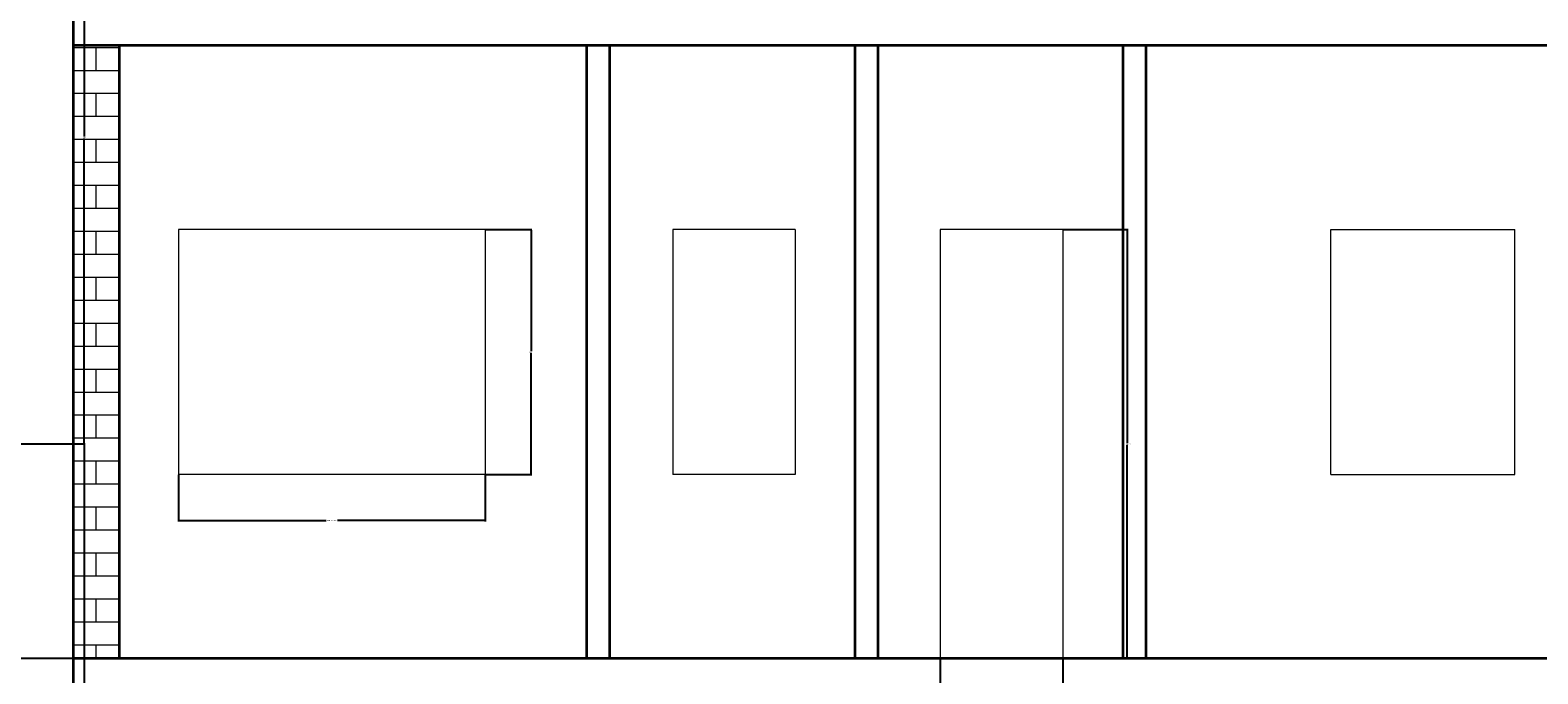
# Model space of a CAD drawing. Units: inches. Extents: x 2120 to 4013, y 1390 to 3019.
# Tile 56 of 59: x 3063 to 3358, y 2598 to 2724. Entities that reach past the tile are written whole.
import ezdxf

# ---------------------------------------------------------------- set-up
doc = ezdxf.new("R2010")
doc.units = ezdxf.units.IN
for name, color, linetype, lineweight in [('A-ANNO-DIMS', 2, 'Continuous', 18), ('A-DOOR', 3, 'Continuous', 18), ('A-GLAZ', 4, 'Continuous', 18), ('A-SECT', 7, 'Continuous', 35), ('A-WALL-PATT', 252, 'Continuous', 13)]:
    doc.layers.add(name, color=color, linetype=linetype, lineweight=lineweight)
doc.styles.get("Standard").update_dxf_attribs({"font": 'arial.ttf'})
doc.dimstyles.get("Standard").update_dxf_attribs({"dimtxt": 0.18, "dimasz": 0.18, "dimexe": 0.18, "dimexo": 0.0625, "dimgap": 0.09, "dimtad": 0, "dimtih": 1, "dimtoh": 1, "dimdec": 4, "dimzin": 0, "dimdsep": 46, "dimtxsty": 'Standard', "dimcen": 0.09, "dimadec": 0, "dimazin": 0, "dimtfac": 1, "dimtdec": 4, "dimtofl": 0, "dimtmove": 0, "dimatfit": 3, "dimfxl": 1, "dimtolj": 1, "dimtzin": 0, "dimarcsym": 0})

# ---------------------------------------------------------------- blocks, each defined once
blk = doc.blocks.new('WIN-SECT-60IN')
for p, q in [((0, 48), (0, 0)), ((60, 48), (0, 48)), ((60, 48), (60, 0)), ((60, 0), (0, 0))]:
    blk.add_line(p, q)
blk = doc.blocks.new('WIN-SECT-24IN')
for p, q in [((0, 48), (0, 0)), ((0, 48), (0, 0)), ((24, 48), (0, 48)), ((24, 48), (24, 0)), ((24, 0), (0, 0))]:
    blk.add_line(p, q)
blk = doc.blocks.new('DOOR-SECT-24IN')
for p, q in [((0, 84), (0, 0)), ((24, 84), (0, 84)), ((24, 84), (24, 0))]:
    blk.add_line(p, q)
blk = doc.blocks.new('WIN-SECT-36IN')
for p, q in [((0, 48), (0, 0)), ((36, 48), (0, 48)), ((36, 48), (36, 0)), ((36, 0), (0, 0))]:
    blk.add_line(p, q)
blk = doc.blocks.new('*D197')
at = {"layer": 'A-ANNO-DIMS', "color": 0, "lineweight": -2, "transparency": 16777216}
for p, q in [((3092.38, 2637.25), (3092.38, 2628.13)), ((3152.38, 2637.25), (3152.38, 2628.13)), ((3092.56, 2628.31), (3121.26, 2628.31)), ((3152.2, 2628.31), (3123.5, 2628.31))]:
    blk.add_line(p, q, dxfattribs=at)
at = {"layer": 'A-ANNO-DIMS', "color": 0, "transparency": 16777216}
for points in [[(3092.56, 2628.34), (3092.56, 2628.28), (3092.38, 2628.31)], [(3152.2, 2628.34), (3152.2, 2628.28), (3152.38, 2628.31)]]:
    blk.add_solid(points, dxfattribs=at)
at = {"layer": 'Defpoints', "color": 0, "transparency": 16777216}
for p in [(3092.38, 2637.31), (3152.38, 2637.31), (3152.38, 2628.31)]:
    blk.add_point(p, dxfattribs=at)
at = {"layer": 'A-ANNO-DIMS', "color": 0, "transparency": 16777216, "insert": (3122.38, 2628.31), "char_height": 0.18, "attachment_point": 5}
blk.add_mtext('\\A1;WINDOW 60 TYP.', dxfattribs=at)
blk = doc.blocks.new('*D198')
at = {"layer": 'A-ANNO-DIMS', "color": 0, "lineweight": -2, "transparency": 16777216}
for p, q in [((3152.44, 2685.31), (3161.56, 2685.31)), ((3161.38, 2685.13), (3161.38, 2661.49)), ((3161.38, 2637.49), (3161.38, 2661.13)), ((3152.44, 2637.31), (3161.56, 2637.31))]:
    blk.add_line(p, q, dxfattribs=at)
at = {"layer": 'A-ANNO-DIMS', "color": 0, "transparency": 16777216}
for points in [[(3161.35, 2685.13), (3161.41, 2685.13), (3161.38, 2685.31)], [(3161.35, 2637.49), (3161.41, 2637.49), (3161.38, 2637.31)]]:
    blk.add_solid(points, dxfattribs=at)
at = {"layer": 'Defpoints', "color": 0, "transparency": 16777216}
for p in [(3152.38, 2685.31), (3161.38, 2685.31), (3152.38, 2637.31)]:
    blk.add_point(p, dxfattribs=at)
at = {"layer": 'A-ANNO-DIMS', "color": 0, "transparency": 16777216, "insert": (3161.38, 2661.31), "char_height": 0.18, "attachment_point": 5}
blk.add_mtext('\\A1;48 TYP.', dxfattribs=at)
blk = doc.blocks.new('*D203')
at = {"layer": 'A-ANNO-DIMS', "color": 0, "lineweight": -2, "transparency": 16777216}
for p, q in [((3265.5, 2685.31), (3278.22, 2685.31)), ((3278.04, 2685.13), (3278.04, 2643.49)), ((3278.04, 2601.49), (3278.04, 2643.13)), ((3265.5, 2601.31), (3278.22, 2601.31))]:
    blk.add_line(p, q, dxfattribs=at)
at = {"layer": 'A-ANNO-DIMS', "color": 0, "transparency": 16777216}
for points in [[(3278.01, 2685.13), (3278.07, 2685.13), (3278.04, 2685.31)], [(3278.01, 2601.49), (3278.07, 2601.49), (3278.04, 2601.31)]]:
    blk.add_solid(points, dxfattribs=at)
at = {"layer": 'Defpoints', "color": 0, "transparency": 16777216}
for p in [(3265.44, 2685.31), (3278.04, 2685.31), (3265.44, 2601.31)]:
    blk.add_point(p, dxfattribs=at)
at = {"layer": 'A-ANNO-DIMS', "color": 0, "transparency": 16777216, "insert": (3278.04, 2643.31), "char_height": 0.18, "attachment_point": 5}
blk.add_mtext('\\A1;DOOR 84 TYP.', dxfattribs=at)
blk = doc.blocks.new('*D204')
at = {"layer": 'A-ANNO-DIMS', "color": 0, "lineweight": -2, "transparency": 16777216}
for p, q in [((3241.44, 2601.25), (3241.44, 2588.53)), ((3265.44, 2601.25), (3265.44, 2588.53)), ((3241.62, 2588.71), (3252.91, 2588.71)), ((3265.26, 2588.71), (3253.97, 2588.71))]:
    blk.add_line(p, q, dxfattribs=at)
at = {"layer": 'A-ANNO-DIMS', "color": 0, "transparency": 16777216}
for points in [[(3241.62, 2588.74), (3241.62, 2588.68), (3241.44, 2588.71)], [(3265.26, 2588.74), (3265.26, 2588.68), (3265.44, 2588.71)]]:
    blk.add_solid(points, dxfattribs=at)
at = {"layer": 'Defpoints', "color": 0, "transparency": 16777216}
for p in [(3241.44, 2601.31), (3265.44, 2601.31), (3265.44, 2588.71)]:
    blk.add_point(p, dxfattribs=at)
at = {"layer": 'A-ANNO-DIMS', "color": 0, "transparency": 16777216, "insert": (3253.44, 2588.71), "char_height": 0.18, "attachment_point": 5}
blk.add_mtext('\\A1;24 TYP.', dxfattribs=at)
blk = doc.blocks.new('*D234')
at = {"layer": 'A-ANNO-DIMS', "color": 0, "lineweight": -2, "transparency": 16777216}
for p, q in [((3033.8, 2643.31), (3074.11, 2643.31)), ((3073.93, 2643.13), (3073.93, 2583.49)), ((3073.93, 2523.49), (3073.93, 2583.13)), ((3009.8, 2523.31), (3074.11, 2523.31))]:
    blk.add_line(p, q, dxfattribs=at)
at = {"layer": 'A-ANNO-DIMS', "color": 0, "transparency": 16777216}
for points in [[(3073.9, 2643.13), (3073.96, 2643.13), (3073.93, 2643.31)], [(3073.9, 2523.49), (3073.96, 2523.49), (3073.93, 2523.31)]]:
    blk.add_solid(points, dxfattribs=at)
at = {"layer": 'Defpoints', "color": 0, "transparency": 16777216}
for p in [(3033.73, 2643.31), (3073.93, 2643.31), (3009.73, 2523.31)]:
    blk.add_point(p, dxfattribs=at)
at = {"layer": 'A-ANNO-DIMS', "color": 0, "transparency": 16777216, "insert": (3073.93, 2583.31), "char_height": 0.18, "attachment_point": 5}
blk.add_mtext('\\A1;120', dxfattribs=at)
blk = doc.blocks.new('*D235')
at = {"layer": 'A-ANNO-DIMS', "color": 0, "lineweight": -2, "transparency": 16777216}
for p, q in [((3033.8, 2763.31), (3074.11, 2763.31)), ((3073.93, 2763.13), (3073.93, 2703.49)), ((3073.93, 2643.49), (3073.93, 2703.13)), ((3033.8, 2643.31), (3074.11, 2643.31))]:
    blk.add_line(p, q, dxfattribs=at)
at = {"layer": 'A-ANNO-DIMS', "color": 0, "transparency": 16777216}
for points in [[(3073.9, 2763.13), (3073.96, 2763.13), (3073.93, 2763.31)], [(3073.9, 2643.49), (3073.96, 2643.49), (3073.93, 2643.31)]]:
    blk.add_solid(points, dxfattribs=at)
at = {"layer": 'Defpoints', "color": 0, "transparency": 16777216}
for p in [(3033.73, 2763.31), (3073.93, 2763.31), (3033.73, 2643.31)]:
    blk.add_point(p, dxfattribs=at)
at = {"layer": 'A-ANNO-DIMS', "color": 0, "transparency": 16777216, "insert": (3073.93, 2703.31), "char_height": 0.18, "attachment_point": 5}
blk.add_mtext('\\A1;120', dxfattribs=at)
blk = doc.blocks.new('*D238')
at = {"layer": 'A-ANNO-DIMS', "color": 0, "lineweight": -2, "transparency": 16777216}
for p, q in [((3071.67, 2601.31), (3026.6, 2601.31)), ((3026.78, 2601.13), (3026.78, 2538.49)), ((3026.78, 2475.49), (3026.78, 2538.13)), ((3071.67, 2475.31), (3026.6, 2475.31))]:
    blk.add_line(p, q, dxfattribs=at)
at = {"layer": 'A-ANNO-DIMS', "color": 0, "transparency": 16777216}
for points in [[(3026.75, 2601.13), (3026.81, 2601.13), (3026.78, 2601.31)], [(3026.75, 2475.49), (3026.81, 2475.49), (3026.78, 2475.31)]]:
    blk.add_solid(points, dxfattribs=at)
at = {"layer": 'Defpoints', "color": 0, "transparency": 16777216}
for p in [(3026.78, 2601.31), (3071.73, 2601.31), (3071.73, 2475.31)]:
    blk.add_point(p, dxfattribs=at)
at = {"layer": 'A-ANNO-DIMS', "color": 0, "transparency": 16777216, "insert": (3026.78, 2538.31), "char_height": 0.18, "attachment_point": 5}
blk.add_mtext('\\A1;126', dxfattribs=at)
blk = doc.blocks.new('*D239')
at = {"layer": 'A-ANNO-DIMS', "color": 0, "lineweight": -2, "transparency": 16777216}
for p, q in [((3071.67, 2727.31), (3026.6, 2727.31)), ((3026.78, 2727.13), (3026.78, 2664.49)), ((3026.78, 2601.49), (3026.78, 2664.13)), ((3071.67, 2601.31), (3026.6, 2601.31))]:
    blk.add_line(p, q, dxfattribs=at)
at = {"layer": 'A-ANNO-DIMS', "color": 0, "transparency": 16777216}
for points in [[(3026.75, 2727.13), (3026.81, 2727.13), (3026.78, 2727.31)], [(3026.75, 2601.49), (3026.81, 2601.49), (3026.78, 2601.31)]]:
    blk.add_solid(points, dxfattribs=at)
at = {"layer": 'Defpoints', "color": 0, "transparency": 16777216}
for p in [(3026.78, 2727.31), (3071.73, 2727.31), (3071.73, 2601.31)]:
    blk.add_point(p, dxfattribs=at)
at = {"layer": 'A-ANNO-DIMS', "color": 0, "transparency": 16777216, "insert": (3026.78, 2664.31), "char_height": 0.18, "attachment_point": 5}
blk.add_mtext('\\A1;126', dxfattribs=at)

msp = doc.modelspace()

# ---------------------------------------------------------------- hatches: boundary and pattern name
at = {"layer": 'A-WALL-PATT'}
h = msp.add_hatch(dxfattribs=at)
h.set_pattern_fill('BRICK', color=256, scale=0.708254, style=0)
h.paths.add_polyline_path([(3071.7347, 2601.3118), (3080.7347, 2601.3118), (3080.7347, 2721.3118), (3071.7347, 2721.3118)])

# ---------------------------------------------------------------- linework, layer by layer
at = {"layer": 'A-SECT'}
for p, q in [((3071.7347, 2895.3118), (3071.7347, 2709.3118)), ((3071.7347, 2769.3118), (3071.7347, 2583.3118)), ((3446.7347, 2721.3118), (3071.7347, 2721.3118)), ((3080.7347, 2721.3118), (3080.7347, 2601.3118)), ((3172.2347, 2721.3118), (3172.2347, 2601.3118)), ((3176.7347, 2721.3118), (3176.7347, 2601.3118)), ((3224.7347, 2721.3118), (3224.7347, 2601.3118)), ((3224.7347, 2721.3118), (3224.7347, 2601.3118)), ((3229.2347, 2721.3118), (3229.2347, 2601.3118)), ((3277.2347, 2721.3118), (3277.2347, 2601.3118)), ((3281.7347, 2721.3118), (3281.7347, 2601.3118)), ((3071.7347, 2643.3118), (3071.7347, 2469.3118)), ((3446.7347, 2601.3118), (3071.7347, 2601.3118))]:
    msp.add_line(p, q, dxfattribs=at)

# ---------------------------------------------------------------- block references
at = {"layer": 'A-DOOR'}
msp.add_blockref('DOOR-SECT-24IN', (3241.4354, 2601.3118), dxfattribs=at)
at = {"layer": 'A-GLAZ'}
for name, p in [('WIN-SECT-60IN', (3092.3803, 2637.3118)), ('WIN-SECT-24IN', (3189.0958, 2637.3118))]:
    msp.add_blockref(name, p, dxfattribs=at)
at = {"layer": 'A-GLAZ', "rotation": 180}
msp.add_blockref('WIN-SECT-36IN', (3353.9131, 2685.3118), dxfattribs=at)

# ---------------------------------------------------------------- dimensions: what is measured, and where the dimension line sits
at = {"layer": 'A-ANNO-DIMS'}
for base, p1, p2, picture, middle in [((3073.9331, 2763.3118), (3033.7331, 2643.3118), (3033.7331, 2763.3118), '*D235', (3073.9331, 2703.3118)), ((3026.7847, 2727.3118), (3071.7347, 2601.3118), (3071.7347, 2727.3118), '*D239', (3026.7847, 2664.3118)), ((3073.9331, 2643.3118), (3009.7331, 2523.3118), (3033.7331, 2643.3118), '*D234', (3073.9331, 2583.3118)), ((3026.7847, 2601.3118), (3071.7347, 2475.3118), (3071.7347, 2601.3118), '*D238', (3026.7847, 2538.3118))]:
    dim = msp.add_linear_dim(base=base, p1=p1, p2=p2, angle=90, dimstyle='Standard', override={"dimdec": 0, "dimlfac": 1, "dimrnd": 0, "dimzin": 0, "dimdsep": 46, "dimlunit": 2}, dxfattribs=at)
    dim.commit()
    dim.dimension.update_dxf_attribs({"geometry": picture, "text_midpoint": middle})
for base, p1, p2, text, picture, middle in [((3161.3803, 2685.3118), (3152.3803, 2637.3118), (3152.3803, 2685.3118), '<> TYP.', '*D198', (3161.3803, 2661.3118)), ((3278.0354, 2685.3118), (3265.4354, 2601.3118), (3265.4354, 2685.3118), 'DOOR <> TYP.', '*D203', (3278.0354, 2643.3118))]:
    dim = msp.add_linear_dim(base=base, p1=p1, p2=p2, angle=90, text=text, dimstyle='Standard', override={"dimdec": 0, "dimlfac": 1, "dimrnd": 0, "dimzin": 0, "dimdsep": 46, "dimlunit": 2}, dxfattribs=at)
    dim.commit()
    dim.dimension.update_dxf_attribs({"geometry": picture, "text_midpoint": middle})
for base, p1, p2, text, picture, middle in [((3152.3803, 2628.3118), (3092.3803, 2637.3118), (3152.3803, 2637.3118), 'WINDOW <> TYP.', '*D197', (3122.3803, 2628.3118)), ((3265.4354, 2588.7118), (3241.4354, 2601.3118), (3265.4354, 2601.3118), '<> TYP.', '*D204', (3253.4354, 2588.7118))]:
    dim = msp.add_linear_dim(base=base, p1=p1, p2=p2, text=text, dimstyle='Standard', override={"dimdec": 0, "dimlfac": 1, "dimrnd": 0, "dimzin": 0, "dimdsep": 46, "dimlunit": 2}, dxfattribs=at)
    dim.commit()
    dim.dimension.update_dxf_attribs({"geometry": picture, "text_midpoint": middle})

doc.saveas('drawing.dxf')
